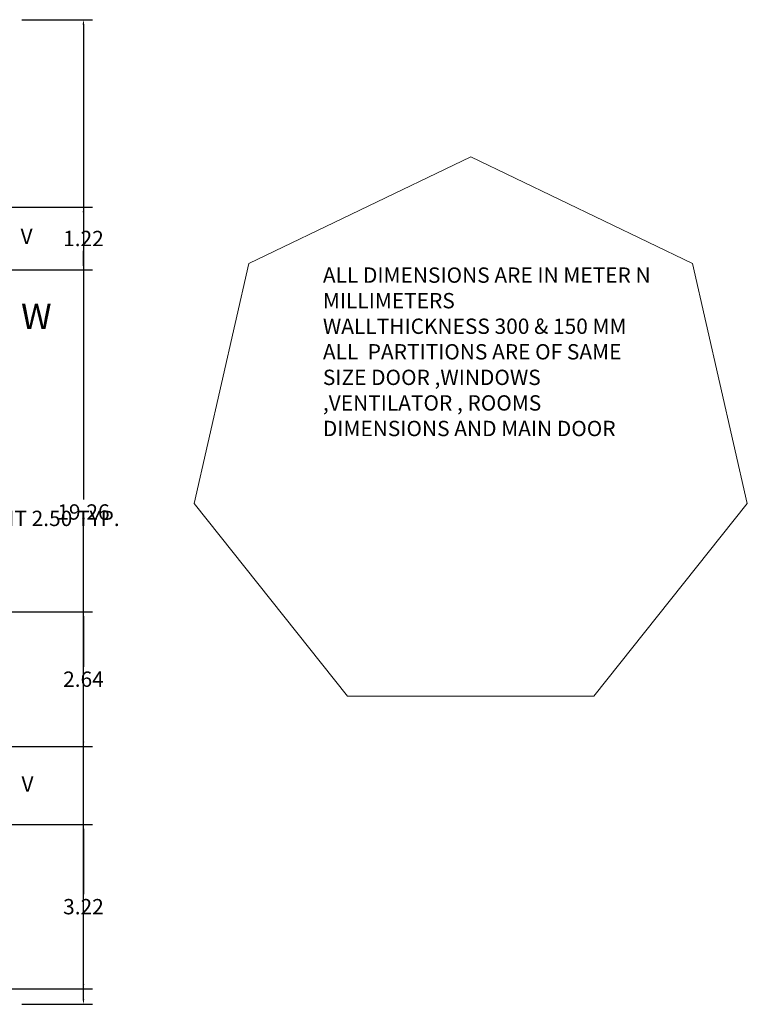
# Model space of a CAD drawing. Units: metres. Extents: x 11 to 49.6, y -23.3 to -0.8.
# Tile 5 of 5: x 35.3 to 49.6, y -21.8 to -2.6. Entities that reach past the tile are written whole.
import ezdxf

# ---------------------------------------------------------------- set-up
doc = ezdxf.new("R2010")
doc.units = ezdxf.units.M
doc.header["$MEASUREMENT"] = 0
for name, color, linetype, lineweight in [('A-ANNO-DIMS', 2, 'Continuous', 18), ('A-ANNO-IDEN', 3, 'Continuous', 18), ('A-ANNO-TEXT', 7, 'Continuous', 18)]:
    doc.layers.add(name, color=color, linetype=linetype, lineweight=lineweight)
doc.styles.get("Standard").update_dxf_attribs({"font": 'arial.ttf'})
doc.dimstyles.get("Standard").update_dxf_attribs({"dimtxt": 0.3, "dimasz": 0.1, "dimexe": 0.18, "dimexo": 0.0625, "dimgap": 0.09, "dimtad": 0, "dimtih": 1, "dimtoh": 1, "dimzin": 0, "dimdsep": 46, "dimtxsty": 'Standard', "dimcen": 0.09, "dimadec": 0, "dimazin": 0, "dimtfac": 1, "dimtofl": 0, "dimtmove": 0, "dimatfit": 3, "dimfxl": 1, "dimtolj": 1, "dimtzin": 0, "dimarcsym": 0})

# ---------------------------------------------------------------- blocks, each defined once
blk = doc.blocks.new('*D54')
at = {"layer": 'A-ANNO-DIMS', "color": 0, "lineweight": -2, "transparency": 16777216}
for p, q in [((31.289, -12.654), (31.289, -12.161)), ((33.789, -12.654), (33.789, -12.161)), ((31.389, -12.341), (33.689, -12.341)), ((33.789, -12.341), (33.889, -12.341))]:
    blk.add_line(p, q, dxfattribs=at)
at = {"layer": 'A-ANNO-DIMS', "color": 0, "transparency": 16777216}
for points in [[(31.389, -12.324), (31.389, -12.358), (31.289, -12.341)], [(33.689, -12.324), (33.689, -12.358), (33.789, -12.341)]]:
    blk.add_solid(points, dxfattribs=at)
at = {"layer": 'Defpoints', "color": 0, "transparency": 16777216}
for p in [(33.789, -12.341), (31.289, -12.716), (33.789, -12.716)]:
    blk.add_point(p, dxfattribs=at)
at = {"layer": 'A-ANNO-DIMS', "color": 0, "transparency": 16777216, "insert": (35.679, -12.341), "char_height": 0.3, "attachment_point": 5}
blk.add_mtext('\\A1;FLIGHT 2.50 TYP.', dxfattribs=at)
blk = doc.blocks.new('*D56')
at = {"layer": 'A-ANNO-DIMS', "color": 0, "lineweight": -2, "transparency": 16777216}
for p, q in [((35.372, -2.586), (36.754, -2.586)), ((36.574, -2.686), (36.574, -11.973)), ((36.574, -21.746), (36.574, -12.459)), ((35.372, -21.846), (36.754, -21.846))]:
    blk.add_line(p, q, dxfattribs=at)
at = {"layer": 'A-ANNO-DIMS', "color": 0, "transparency": 16777216}
for points in [[(36.558, -2.686), (36.591, -2.686), (36.574, -2.586)], [(36.558, -21.746), (36.591, -21.746), (36.574, -21.846)]]:
    blk.add_solid(points, dxfattribs=at)
at = {"layer": 'Defpoints', "color": 0, "transparency": 16777216}
for p in [(35.309, -2.586), (35.309, -21.846), (36.574, -21.846)]:
    blk.add_point(p, dxfattribs=at)
at = {"layer": 'A-ANNO-DIMS', "color": 0, "transparency": 16777216, "insert": (36.574, -12.216), "char_height": 0.3, "attachment_point": 5}
blk.add_mtext('\\A1;19.26', dxfattribs=at)
blk = doc.blocks.new('*D58')
at = {"layer": 'A-ANNO-DIMS', "color": 0, "lineweight": -2, "transparency": 16777216}
for p, q in [((32.672, -6.256), (36.754, -6.256)), ((36.574, -6.356), (36.574, -6.625)), ((36.574, -7.376), (36.574, -7.107)), ((32.672, -7.476), (36.754, -7.476))]:
    blk.add_line(p, q, dxfattribs=at)
at = {"layer": 'A-ANNO-DIMS', "color": 0, "transparency": 16777216}
for points in [[(36.558, -6.356), (36.591, -6.356), (36.574, -6.256)], [(36.558, -7.376), (36.591, -7.376), (36.574, -7.476)]]:
    blk.add_solid(points, dxfattribs=at)
at = {"layer": 'Defpoints', "color": 0, "transparency": 16777216}
for p in [(32.609, -6.256), (32.609, -7.476), (36.574, -7.476)]:
    blk.add_point(p, dxfattribs=at)
at = {"layer": 'A-ANNO-DIMS', "color": 0, "transparency": 16777216, "insert": (36.574, -6.866), "char_height": 0.3, "attachment_point": 5}
blk.add_mtext('\\A1;1.22', dxfattribs=at)
blk = doc.blocks.new('*D71')
at = {"layer": 'A-ANNO-DIMS', "color": 0, "lineweight": -2, "transparency": 16777216}
for p, q in [((23.641, -14.166), (36.754, -14.166)), ((36.574, -14.266), (36.574, -15.243)), ((36.574, -16.706), (36.574, -15.729)), ((23.641, -16.806), (36.754, -16.806))]:
    blk.add_line(p, q, dxfattribs=at)
at = {"layer": 'A-ANNO-DIMS', "color": 0, "transparency": 16777216}
for points in [[(36.558, -14.266), (36.591, -14.266), (36.574, -14.166)], [(36.558, -16.706), (36.591, -16.706), (36.574, -16.806)]]:
    blk.add_solid(points, dxfattribs=at)
at = {"layer": 'Defpoints', "color": 0, "transparency": 16777216}
for p in [(23.579, -14.166), (23.579, -16.806), (36.574, -16.806)]:
    blk.add_point(p, dxfattribs=at)
at = {"layer": 'A-ANNO-DIMS', "color": 0, "transparency": 16777216, "insert": (36.574, -15.486), "char_height": 0.3, "attachment_point": 5}
blk.add_mtext('\\A1;2.64', dxfattribs=at)
blk = doc.blocks.new('*D72')
at = {"layer": 'A-ANNO-DIMS', "color": 0, "lineweight": -2, "transparency": 16777216}
for p, q in [((23.491, -18.326), (36.754, -18.326)), ((36.574, -18.426), (36.574, -19.693)), ((36.574, -21.446), (36.574, -20.179)), ((23.491, -21.546), (36.754, -21.546))]:
    blk.add_line(p, q, dxfattribs=at)
at = {"layer": 'A-ANNO-DIMS', "color": 0, "transparency": 16777216}
for points in [[(36.558, -18.426), (36.591, -18.426), (36.574, -18.326)], [(36.558, -21.446), (36.591, -21.446), (36.574, -21.546)]]:
    blk.add_solid(points, dxfattribs=at)
at = {"layer": 'Defpoints', "color": 0, "transparency": 16777216}
for p in [(23.429, -18.326), (23.429, -21.546), (36.574, -21.546)]:
    blk.add_point(p, dxfattribs=at)
at = {"layer": 'A-ANNO-DIMS', "color": 0, "transparency": 16777216, "insert": (36.574, -19.936), "char_height": 0.3, "attachment_point": 5}
blk.add_mtext('\\A1;3.22', dxfattribs=at)

msp = doc.modelspace()

# ---------------------------------------------------------------- linework, layer by layer
at = {"layer": 'A-ANNO-TEXT'}
msp.add_lwpolyline([(44.15, -5.268), (39.811, -7.357), (38.739, -12.052), (41.742, -15.817), (46.557, -15.817), (49.56, -12.052), (48.488, -7.357)], close=True, dxfattribs=at)

# ---------------------------------------------------------------- texts
at = {"layer": 'A-ANNO-IDEN', "attachment_point": 1}
for s, width, insert, char_height in [('V', 0.1, (35.344, -6.672), 0.3), ('W', 1.41386, (35.353, -8.139), 0.5), ('V', 0.1, (35.362, -17.387), 0.3)]:
    msp.add_mtext_dynamic_manual_height_columns(s, width=width, gutter_width=0.5, heights=[0], dxfattribs=dict(at, insert=insert, char_height=char_height))
at = {"layer": 'A-ANNO-TEXT', "insert": (41.258, -7.432), "char_height": 0.3, "attachment_point": 1}
msp.add_mtext_dynamic_manual_height_columns('ALL DIMENSIONS ARE IN METER N MILLIMETERS \\PWALLTHICKNESS 300 & 150 MM \\PALL  PARTITIONS ARE OF SAME SIZE DOOR ,WINDOWS ,VENTILATOR , ROOMS DIMENSIONS AND MAIN DOOR ', width=6.70255, gutter_width=0.5, heights=[0], dxfattribs=at)

# ---------------------------------------------------------------- dimensions: what is measured, and where the dimension line sits
at = {"layer": 'A-ANNO-DIMS'}
for base, p1, p2, picture, middle in [((36.574, -21.846), (35.309, -2.586), (35.309, -21.846), '*D56', (36.574, -12.216)), ((36.574, -7.476), (32.609, -6.256), (32.609, -7.476), '*D58', (36.574, -6.866)), ((36.574, -16.806), (23.579, -14.166), (23.579, -16.806), '*D71', (36.574, -15.486)), ((36.574, -21.546), (23.429, -18.326), (23.429, -21.546), '*D72', (36.574, -19.936))]:
    dim = msp.add_linear_dim(base=base, p1=p1, p2=p2, angle=90, dimstyle='Standard', override={"dimdec": 2, "dimlfac": 1, "dimrnd": 0, "dimzin": 0, "dimdsep": 46, "dimlunit": 2}, dxfattribs=at)
    dim.commit()
    dim.dimension.update_dxf_attribs({"geometry": picture, "text_midpoint": middle})
dim = msp.add_linear_dim(base=(33.789, -12.341), p1=(31.289, -12.716), p2=(33.789, -12.716), text='FLIGHT <> TYP.', dimstyle='Standard', override={"dimdec": 2, "dimlfac": 1, "dimrnd": 0, "dimzin": 0, "dimdsep": 46, "dimlunit": 2}, dxfattribs=at)
dim.commit()
dim.dimension.update_dxf_attribs({"geometry": '*D54', "text_midpoint": (35.679, -12.341)})

doc.saveas('drawing.dxf')
